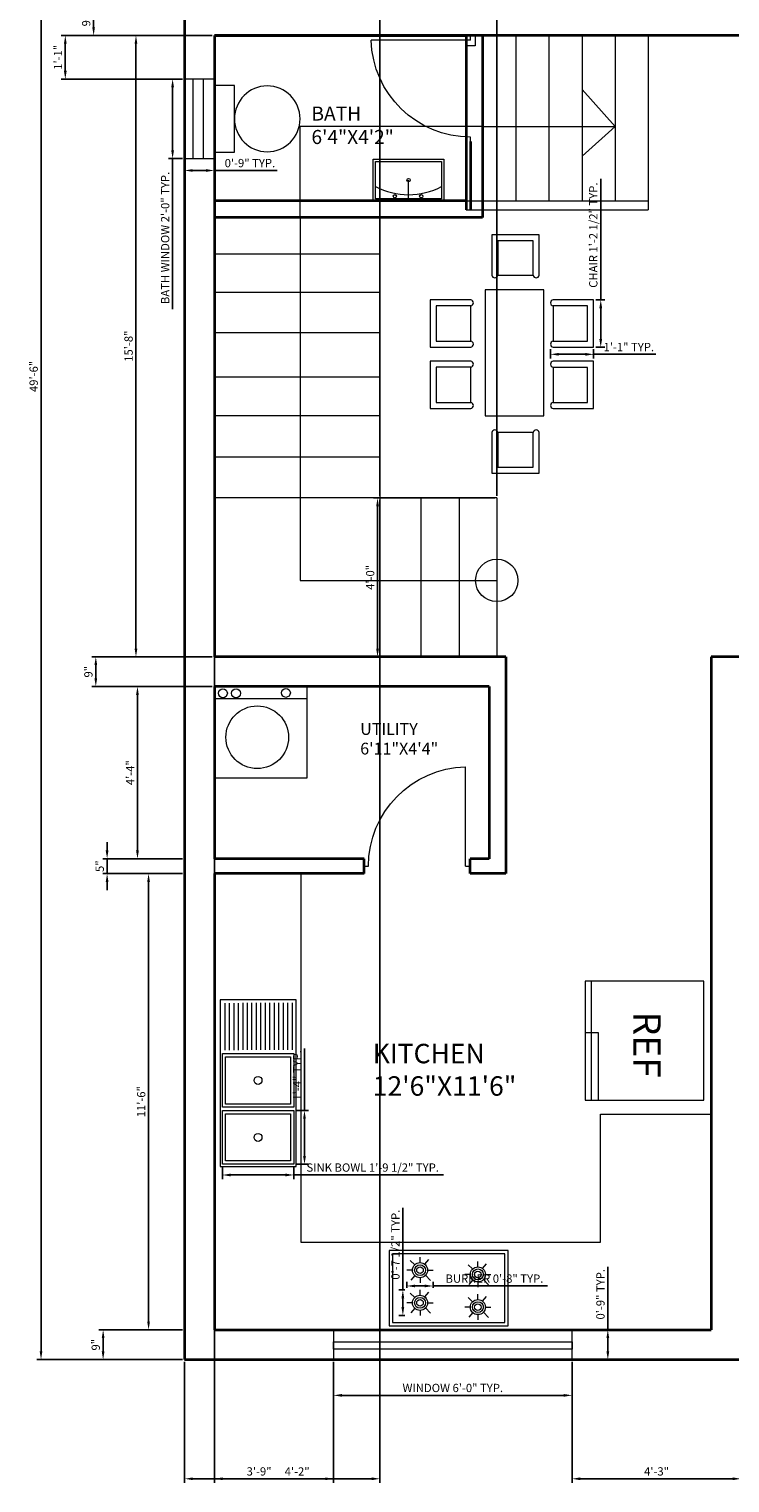
# Model space of a CAD drawing. Units: inches. Extents: x 808 to 1433, y 803 to 1556.
# Tile 1 of 4: x 808 to 1020, y 804 to 1243. Entities that reach past the tile are written whole.
import ezdxf

# ---------------------------------------------------------------- set-up
doc = ezdxf.new("R2010")
doc.units = ezdxf.units.IN
for name, color, linetype, lineweight in [('A-ANNO-DIMS', 7, 'Continuous', 13), ('A-AREA-IDEN', 7, 'Continuous', 18), ('A-FLOR-CASE', 7, 'Continuous', 18), ('A-FLOR-STRS', 7, 'Continuous', 18), ('A-WALL', 7, 'Continuous', 35)]:
    doc.layers.add(name, color=color, linetype=linetype, lineweight=lineweight)
for name, color, linetype, lineweight, true_color in [('A-ANNO-TEXT', 251, 'Continuous', 18, 0x636466), ('A-DOOR', 251, 'Continuous', 18, 0x636466), ('A-EQPM', 251, 'Continuous', 18, 0x636466), ('A-FIXT-PATT', 251, 'Continuous', 13, 0x636466), ('A-FLOR-FIXT', 251, 'Continuous', 18, 0x636466), ('A-FURN', 251, 'Continuous', 13, 0x636466), ('A-GLAZ', 251, 'Continuous', 18, 0x636466)]:
    doc.layers.add(name, color=color, linetype=linetype, lineweight=lineweight, true_color=true_color)
doc.styles.get("Standard").update_dxf_attribs({"font": 'arial.ttf'})
doc.dimstyles.new('ISO-25', dxfattribs={"dimtxt": 2.5, "dimasz": 2.5, "dimexe": 1.25, "dimexo": 0.625, "dimtad": 1, "dimdec": 0, "dimlunit": 3, "dimtxsty": 'Standard', "dimcen": 2.5, "dimadec": 0, "dimazin": 0, "dimtfac": 1, "dimtdec": 0, "dimtmove": 0, "dimatfit": 3, "dimfxl": 1, "dimarcsym": 0})

# ---------------------------------------------------------------- blocks, each defined once
blk = doc.blocks.new('*D12')
at = {"layer": 'A-ANNO-DIMS', "color": 0, "lineweight": -2, "transparency": 16777216}
for p, q in [((854.25, 1435.07), (810.3, 1435.07)), ((811.55, 1432.57), (811.55, 843.57)), ((854.25, 841.07), (810.3, 841.07))]:
    blk.add_line(p, q, dxfattribs=at)
at = {"layer": 'A-ANNO-DIMS', "color": 0, "transparency": 16777216}
for points in [[(811.14, 1432.57), (811.97, 1432.57), (811.55, 1435.07)], [(811.14, 843.57), (811.97, 843.57), (811.55, 841.07)]]:
    blk.add_solid(points, dxfattribs=at)
at = {"layer": 'Defpoints', "color": 0, "transparency": 16777216}
for p in [(854.88, 1435.07), (811.55, 841.07), (854.88, 841.07)]:
    blk.add_point(p, dxfattribs=at)
at = {"layer": 'A-ANNO-DIMS', "color": 0, "transparency": 16777216, "insert": (809.65, 1138.07), "char_height": 2.5, "attachment_point": 5, "rotation": 90}
blk.add_mtext('49\'-6"', dxfattribs=at)
blk = doc.blocks.new('*D15')
at = {"layer": 'A-ANNO-DIMS', "color": 0, "lineweight": -2, "transparency": 16777216}
for p, q in [((854.25, 1250.07), (826.18, 1250.07)), ((827.43, 1247.57), (827.43, 1243.57)), ((854.25, 1241.07), (826.18, 1241.07))]:
    blk.add_line(p, q, dxfattribs=at)
at = {"layer": 'A-ANNO-DIMS', "color": 0, "transparency": 16777216}
for points in [[(827.01, 1247.57), (827.84, 1247.57), (827.43, 1250.07)], [(827.01, 1243.57), (827.84, 1243.57), (827.43, 1241.07)]]:
    blk.add_solid(points, dxfattribs=at)
at = {"layer": 'Defpoints', "color": 0, "transparency": 16777216}
for p in [(854.88, 1250.07), (827.43, 1241.07), (854.88, 1241.07)]:
    blk.add_point(p, dxfattribs=at)
at = {"layer": 'A-ANNO-DIMS', "color": 0, "transparency": 16777216, "insert": (825.52, 1245.57), "char_height": 2.5, "attachment_point": 5, "rotation": 90}
blk.add_mtext('9"', dxfattribs=at)
blk = doc.blocks.new('*D16')
at = {"layer": 'A-ANNO-DIMS', "color": 0, "lineweight": -2, "transparency": 16777216}
for p, q in [((854.25, 1044.37), (839.42, 1044.37)), ((840.67, 1041.87), (840.67, 994.87)), ((854.25, 992.37), (839.42, 992.37))]:
    blk.add_line(p, q, dxfattribs=at)
at = {"layer": 'A-ANNO-DIMS', "color": 0, "transparency": 16777216}
for points in [[(840.25, 1041.87), (841.08, 1041.87), (840.67, 1044.37)], [(840.25, 994.87), (841.08, 994.87), (840.67, 992.37)]]:
    blk.add_solid(points, dxfattribs=at)
at = {"layer": 'Defpoints', "color": 0, "transparency": 16777216}
for p in [(854.88, 1044.37), (840.67, 992.37), (854.88, 992.37)]:
    blk.add_point(p, dxfattribs=at)
at = {"layer": 'A-ANNO-DIMS', "color": 0, "transparency": 16777216, "insert": (838.79, 1018.37), "char_height": 2.5, "attachment_point": 5, "rotation": 90}
blk.add_mtext('4\'-4"', dxfattribs=at)
blk = doc.blocks.new('*D17')
at = {"layer": 'A-ANNO-DIMS', "color": 0, "lineweight": -2, "transparency": 16777216}
for p, q in [((831.5, 994.87), (831.5, 997.37)), ((854.25, 992.37), (830.25, 992.37)), ((831.5, 992.37), (831.5, 987.87)), ((854.25, 987.87), (830.25, 987.87)), ((831.5, 985.37), (831.5, 982.87))]:
    blk.add_line(p, q, dxfattribs=at)
at = {"layer": 'A-ANNO-DIMS', "color": 0, "transparency": 16777216}
for points in [[(831.08, 994.87), (831.91, 994.87), (831.5, 992.37)], [(831.08, 985.37), (831.91, 985.37), (831.5, 987.87)]]:
    blk.add_solid(points, dxfattribs=at)
at = {"layer": 'Defpoints', "color": 0, "transparency": 16777216}
for p in [(854.88, 992.37), (831.5, 987.87), (854.88, 987.87)]:
    blk.add_point(p, dxfattribs=at)
at = {"layer": 'A-ANNO-DIMS', "color": 0, "transparency": 16777216, "insert": (829.6, 990.12), "char_height": 2.5, "attachment_point": 5, "rotation": 90}
blk.add_mtext('5"', dxfattribs=at)
blk = doc.blocks.new('*D18')
at = {"layer": 'A-ANNO-DIMS', "color": 0, "lineweight": -2, "transparency": 16777216}
for p, q in [((854.25, 987.87), (842.77, 987.87)), ((844.02, 985.37), (844.02, 852.57)), ((854.25, 850.07), (842.77, 850.07))]:
    blk.add_line(p, q, dxfattribs=at)
at = {"layer": 'A-ANNO-DIMS', "color": 0, "transparency": 16777216}
for points in [[(843.6, 985.37), (844.43, 985.37), (844.02, 987.87)], [(843.6, 852.57), (844.43, 852.57), (844.02, 850.07)]]:
    blk.add_solid(points, dxfattribs=at)
at = {"layer": 'Defpoints', "color": 0, "transparency": 16777216}
for p in [(854.88, 987.87), (844.02, 850.07), (854.88, 850.07)]:
    blk.add_point(p, dxfattribs=at)
at = {"layer": 'A-ANNO-DIMS', "color": 0, "transparency": 16777216, "insert": (842.12, 918.97), "char_height": 2.5, "attachment_point": 5, "rotation": 90}
blk.add_mtext('11\'-6"', dxfattribs=at)
blk = doc.blocks.new('*D19')
at = {"layer": 'A-ANNO-DIMS', "color": 0, "lineweight": -2, "transparency": 16777216}
for p, q in [((854.25, 850.07), (829.05, 850.07)), ((830.3, 847.57), (830.3, 843.57)), ((854.25, 841.07), (829.05, 841.07))]:
    blk.add_line(p, q, dxfattribs=at)
at = {"layer": 'A-ANNO-DIMS', "color": 0, "transparency": 16777216}
for points in [[(829.88, 847.57), (830.71, 847.57), (830.3, 850.07)], [(829.88, 843.57), (830.71, 843.57), (830.3, 841.07)]]:
    blk.add_solid(points, dxfattribs=at)
at = {"layer": 'Defpoints', "color": 0, "transparency": 16777216}
for p in [(854.88, 850.07), (830.3, 841.07), (854.88, 841.07)]:
    blk.add_point(p, dxfattribs=at)
at = {"layer": 'A-ANNO-DIMS', "color": 0, "transparency": 16777216, "insert": (828.39, 845.57), "char_height": 2.5, "attachment_point": 5, "rotation": 90}
blk.add_mtext('9"', dxfattribs=at)
blk = doc.blocks.new('*D27')
at = {"layer": 'A-ANNO-DIMS', "color": 0, "lineweight": -2, "transparency": 16777216}
for p, q in [((863.25, 1053.37), (826.84, 1053.37)), ((828.09, 1050.87), (828.09, 1046.87)), ((863.25, 1044.37), (826.84, 1044.37))]:
    blk.add_line(p, q, dxfattribs=at)
at = {"layer": 'A-ANNO-DIMS', "color": 0, "transparency": 16777216}
for points in [[(827.67, 1050.87), (828.5, 1050.87), (828.09, 1053.37)], [(827.67, 1046.87), (828.5, 1046.87), (828.09, 1044.37)]]:
    blk.add_solid(points, dxfattribs=at)
at = {"layer": 'Defpoints', "color": 0, "transparency": 16777216}
for p in [(863.88, 1053.37), (828.09, 1044.37), (863.88, 1044.37)]:
    blk.add_point(p, dxfattribs=at)
at = {"layer": 'A-ANNO-DIMS', "color": 0, "transparency": 16777216, "insert": (826.18, 1048.87), "char_height": 2.5, "attachment_point": 5, "rotation": 90}
blk.add_mtext('9"', dxfattribs=at)
blk = doc.blocks.new('*D28')
at = {"layer": 'A-ANNO-DIMS', "color": 0, "lineweight": -2, "transparency": 16777216}
for p, q in [((854.25, 1241.07), (838.97, 1241.07)), ((840.22, 1055.87), (840.22, 1238.57)), ((854.25, 1053.37), (838.97, 1053.37))]:
    blk.add_line(p, q, dxfattribs=at)
at = {"layer": 'A-ANNO-DIMS', "color": 0, "transparency": 16777216}
for points in [[(839.8, 1238.57), (840.63, 1238.57), (840.22, 1241.07)], [(839.8, 1055.87), (840.63, 1055.87), (840.22, 1053.37)]]:
    blk.add_solid(points, dxfattribs=at)
at = {"layer": 'Defpoints', "color": 0, "transparency": 16777216}
for p in [(840.22, 1241.07), (854.88, 1241.07), (854.88, 1053.37)]:
    blk.add_point(p, dxfattribs=at)
at = {"layer": 'A-ANNO-DIMS', "color": 0, "transparency": 16777216, "insert": (838.31, 1147.22), "char_height": 2.5, "attachment_point": 5, "rotation": 90}
blk.add_mtext('15\'-8"', dxfattribs=at)
blk = doc.blocks.new('WC')
blk.add_lwpolyline([(0, 19.84), (20.21, 19.84), (20.21, 25.9), (0, 25.9)], close=True)
for start, end in [(90, 270), (270, 90)]:
    blk.add_arc((10.11, 9.92), 9.92, start, end)
blk = doc.blocks.new('LAVATORY-COMPACT')
blk.add_line((10.66, 0.67), (10.66, 6.33))
for points in [[(21.33, 0), (0, 0), (0, 12.65), (21.33, 12.65)], [(20.66, 0.67), (0.67, 0.67), (0.67, 11.98), (20.66, 11.98)]]:
    blk.add_lwpolyline(points, close=True)
for centre in [(10.66, 6.33), (6.53, 1.45), (14.51, 1.45)]:
    blk.add_circle(centre, 0.492)
blk.add_arc((10.66, 23.6), 21.69, 242.5485, 297.4515)
blk = doc.blocks.new('COOKTOP-BURNER')
for p, q in [((2.4, 5.45), (1.03, 6.69)), ((3.99, 6.1), (3.99, 7.72)), ((5.4, 5.61), (6.63, 7.04)), ((1.71, 3.81), (0, 3.81)), ((2.42, 2.16), (1.25, 0.81)), ((3.99, 1.53), (3.99, 0)), ((5.67, 2.27), (7.14, 0.65)), ((6.27, 3.81), (7.92, 3.81))]:
    blk.add_line(p, q)
for radius in [2.28, 1.64, 0.989]:
    blk.add_circle((3.99, 3.81), radius)
blk = doc.blocks.new('WIN-72')
for points in [[(0, 0), (72, 0), (72, 9), (0, 9)], [(0, 5.39), (72, 5.39), (72, 3.12), (0, 3.12)]]:
    blk.add_lwpolyline(points, close=True)
blk = doc.blocks.new('WIN-24')
for p, q in [((0, 5.64), (24, 5.64)), ((0, 2.5), (24, 2.5))]:
    blk.add_line(p, q)
blk.add_lwpolyline([(0, 0), (24, 0), (24, 9), (0, 9)], close=True)
blk = doc.blocks.new('DOOR-32')
for p, q in [((1.38, 0), (1.38, 30)), ((1.38, 0), (0, 0)), ((32, 0), (30.69, 0))]:
    blk.add_line(p, q)
blk.add_arc((0.68, 0), 30.01, 0, 88.664)
blk = doc.blocks.new('CHAIR-DINING')
blk.add_lwpolyline([(0.77, 0), (13.02, 0), (13.02, 14.3), (0.77, 14.3)])
blk.add_lwpolyline([(0.77, 1.83), (11.19, 1.83), (11.19, 12.46), (0.77, 12.46)], close=True)
for centre in [(0.93, 13.38), (0.93, 0.92)]:
    blk.add_arc(centre, 0.932, 100.176, 259.824)
blk = doc.blocks.new('SINK-BOWL')
for points in [[(21.57, 0), (0, 0), (0, 16.24), (21.57, 16.24)], [(20.57, 1), (1, 1), (1, 15.24), (20.57, 15.24)]]:
    blk.add_lwpolyline(points, close=True)
blk.add_circle((10.78, 8.12), 1.19)
blk = doc.blocks.new('*D41')
at = {"layer": 'A-ANNO-DIMS', "color": 0, "lineweight": -2, "transparency": 16777216}
for p, q in [((899.87, 840.44), (899.87, 829.02)), ((971.87, 840.44), (971.87, 829.02)), ((902.37, 830.27), (969.37, 830.27))]:
    blk.add_line(p, q, dxfattribs=at)
at = {"layer": 'A-ANNO-DIMS', "color": 0, "transparency": 16777216}
for points in [[(902.37, 830.68), (902.37, 829.85), (899.87, 830.27)], [(969.37, 830.68), (969.37, 829.85), (971.87, 830.27)]]:
    blk.add_solid(points, dxfattribs=at)
at = {"layer": 'Defpoints', "color": 0, "transparency": 16777216}
for p in [(899.87, 841.07), (971.87, 841.07), (971.87, 830.27)]:
    blk.add_point(p, dxfattribs=at)
at = {"layer": 'A-ANNO-DIMS', "color": 0, "transparency": 16777216, "insert": (935.87, 832.18), "char_height": 2.5, "attachment_point": 5}
blk.add_mtext('WINDOW 6\'-0" TYP.', dxfattribs=at)
blk = doc.blocks.new('*D42')
at = {"layer": 'A-ANNO-DIMS', "color": 0, "lineweight": -2, "transparency": 16777216}
for p, q in [((982.67, 850.07), (982.67, 869.05)), ((972.5, 850.07), (983.92, 850.07)), ((982.67, 843.57), (982.67, 847.57)), ((972.5, 841.07), (983.92, 841.07))]:
    blk.add_line(p, q, dxfattribs=at)
at = {"layer": 'A-ANNO-DIMS', "color": 0, "transparency": 16777216}
for points in [[(982.25, 847.57), (983.09, 847.57), (982.67, 850.07)], [(982.25, 843.57), (983.09, 843.57), (982.67, 841.07)]]:
    blk.add_solid(points, dxfattribs=at)
at = {"layer": 'Defpoints', "color": 0, "transparency": 16777216}
for p in [(971.87, 850.07), (982.67, 850.07), (971.87, 841.07)]:
    blk.add_point(p, dxfattribs=at)
at = {"layer": 'A-ANNO-DIMS', "color": 0, "transparency": 16777216, "insert": (980.77, 860.81), "char_height": 2.5, "attachment_point": 5, "rotation": 90}
blk.add_mtext('0\'-9" TYP.', dxfattribs=at)
blk = doc.blocks.new('*D43')
at = {"layer": 'A-ANNO-DIMS', "color": 0, "lineweight": -2, "transparency": 16777216}
for p, q in [((854.25, 1227.89), (850.03, 1227.89)), ((851.28, 1225.39), (851.28, 1206.39)), ((854.25, 1203.89), (850.03, 1203.89)), ((851.28, 1203.89), (851.28, 1158.43))]:
    blk.add_line(p, q, dxfattribs=at)
at = {"layer": 'A-ANNO-DIMS', "color": 0, "transparency": 16777216}
for points in [[(850.86, 1225.39), (851.7, 1225.39), (851.28, 1227.89)], [(850.86, 1206.39), (851.7, 1206.39), (851.28, 1203.89)]]:
    blk.add_solid(points, dxfattribs=at)
at = {"layer": 'Defpoints', "color": 0, "transparency": 16777216}
for p in [(854.88, 1227.89), (851.28, 1203.89), (854.88, 1203.89)]:
    blk.add_point(p, dxfattribs=at)
at = {"layer": 'A-ANNO-DIMS', "color": 0, "transparency": 16777216, "insert": (849.36, 1179.91), "char_height": 2.5, "attachment_point": 5, "rotation": 90}
blk.add_mtext('BATH WINDOW 2\'-0" TYP.', dxfattribs=at)
blk = doc.blocks.new('*D44')
at = {"layer": 'A-ANNO-DIMS', "color": 0, "lineweight": -2, "transparency": 16777216}
for p, q in [((854.88, 1203.26), (854.88, 1199.04)), ((857.38, 1200.29), (861.38, 1200.29)), ((863.88, 1203.26), (863.88, 1199.04)), ((863.88, 1200.29), (882.87, 1200.29))]:
    blk.add_line(p, q, dxfattribs=at)
at = {"layer": 'A-ANNO-DIMS', "color": 0, "transparency": 16777216}
for points in [[(857.38, 1200.7), (857.38, 1199.87), (854.88, 1200.29)], [(861.38, 1200.7), (861.38, 1199.87), (863.88, 1200.29)]]:
    blk.add_solid(points, dxfattribs=at)
at = {"layer": 'Defpoints', "color": 0, "transparency": 16777216}
for p in [(854.88, 1203.89), (863.88, 1203.89), (863.88, 1200.29)]:
    blk.add_point(p, dxfattribs=at)
at = {"layer": 'A-ANNO-DIMS', "color": 0, "transparency": 16777216, "insert": (874.62, 1202.19), "char_height": 2.5, "attachment_point": 5}
blk.add_mtext('0\'-9" TYP.', dxfattribs=at)
blk = doc.blocks.new('*D59')
at = {"layer": 'A-ANNO-DIMS', "color": 0, "lineweight": -2, "transparency": 16777216}
for p, q in [((980.53, 1161.19), (980.53, 1197.81)), ((979.01, 1161.19), (981.78, 1161.19)), ((980.53, 1149.4), (980.53, 1158.69)), ((979.01, 1146.9), (981.78, 1146.9))]:
    blk.add_line(p, q, dxfattribs=at)
at = {"layer": 'A-ANNO-DIMS', "color": 0, "transparency": 16777216}
for points in [[(980.11, 1158.69), (980.95, 1158.69), (980.53, 1161.19)], [(980.11, 1149.4), (980.95, 1149.4), (980.53, 1146.9)]]:
    blk.add_solid(points, dxfattribs=at)
at = {"layer": 'Defpoints', "color": 0, "transparency": 16777216}
for p in [(978.39, 1161.19), (980.53, 1161.19), (978.39, 1146.9)]:
    blk.add_point(p, dxfattribs=at)
at = {"layer": 'A-ANNO-DIMS', "color": 0, "transparency": 16777216, "insert": (978.61, 1180.75), "char_height": 2.5, "attachment_point": 5, "rotation": 90}
blk.add_mtext('CHAIR 1\'-2 1/2" TYP.', dxfattribs=at)
blk = doc.blocks.new('*D60')
at = {"layer": 'A-ANNO-DIMS', "color": 0, "lineweight": -2, "transparency": 16777216}
for p, q in [((965.37, 1146.27), (965.37, 1143.5)), ((967.87, 1144.75), (975.89, 1144.75)), ((978.39, 1146.27), (978.39, 1143.5)), ((978.39, 1144.75), (997.14, 1144.75))]:
    blk.add_line(p, q, dxfattribs=at)
at = {"layer": 'A-ANNO-DIMS', "color": 0, "transparency": 16777216}
for points in [[(967.87, 1145.17), (967.87, 1144.33), (965.37, 1144.75)], [(975.89, 1145.17), (975.89, 1144.33), (978.39, 1144.75)]]:
    blk.add_solid(points, dxfattribs=at)
at = {"layer": 'Defpoints', "color": 0, "transparency": 16777216}
for p in [(965.37, 1146.9), (978.39, 1146.9), (978.39, 1144.75)]:
    blk.add_point(p, dxfattribs=at)
at = {"layer": 'A-ANNO-DIMS', "color": 0, "transparency": 16777216, "insert": (989.01, 1146.63), "char_height": 2.5, "attachment_point": 5}
blk.add_mtext('1\'-1" TYP.', dxfattribs=at)
blk = doc.blocks.new('*D61')
at = {"layer": 'A-ANNO-DIMS', "color": 0, "lineweight": -2, "transparency": 16777216}
for p, q in [((866.29, 899.45), (866.29, 895.59)), ((868.79, 896.84), (885.35, 896.84)), ((887.85, 899.45), (887.85, 895.59)), ((887.85, 896.84), (933.03, 896.84))]:
    blk.add_line(p, q, dxfattribs=at)
at = {"layer": 'A-ANNO-DIMS', "color": 0, "transparency": 16777216}
for points in [[(868.79, 897.26), (868.79, 896.42), (866.29, 896.84)], [(885.35, 897.26), (885.35, 896.42), (887.85, 896.84)]]:
    blk.add_solid(points, dxfattribs=at)
at = {"layer": 'Defpoints', "color": 0, "transparency": 16777216}
for p in [(866.29, 900.07), (887.85, 900.07), (887.85, 896.84)]:
    blk.add_point(p, dxfattribs=at)
at = {"layer": 'A-ANNO-DIMS', "color": 0, "transparency": 16777216, "insert": (911.69, 898.76), "char_height": 2.5, "attachment_point": 5}
blk.add_mtext('SINK BOWL 1\'-9 1/2" TYP.', dxfattribs=at)
blk = doc.blocks.new('*D62')
at = {"layer": 'A-ANNO-DIMS', "color": 0, "lineweight": -2, "transparency": 16777216}
for p, q in [((891.09, 916.31), (891.09, 935.07)), ((888.48, 916.31), (892.34, 916.31)), ((891.09, 902.57), (891.09, 913.81)), ((888.48, 900.07), (892.34, 900.07))]:
    blk.add_line(p, q, dxfattribs=at)
at = {"layer": 'A-ANNO-DIMS', "color": 0, "transparency": 16777216}
for points in [[(890.67, 913.81), (891.51, 913.81), (891.09, 916.31)], [(890.67, 902.57), (891.51, 902.57), (891.09, 900.07)]]:
    blk.add_solid(points, dxfattribs=at)
at = {"layer": 'Defpoints', "color": 0, "transparency": 16777216}
for p in [(887.85, 916.31), (891.09, 916.31), (887.85, 900.07)]:
    blk.add_point(p, dxfattribs=at)
at = {"layer": 'A-ANNO-DIMS', "color": 0, "transparency": 16777216, "insert": (889.21, 926.94), "char_height": 2.5, "attachment_point": 5, "rotation": 90}
blk.add_mtext('1\'-4" TYP.', dxfattribs=at)
blk = doc.blocks.new('*D63')
at = {"layer": 'A-ANNO-DIMS', "color": 0, "lineweight": -2, "transparency": 16777216}
for p, q in [((921.98, 862.75), (921.98, 864.56)), ((924.48, 863.31), (927.4, 863.31)), ((929.9, 862.75), (929.9, 864.56)), ((929.9, 863.31), (964.49, 863.31))]:
    blk.add_line(p, q, dxfattribs=at)
at = {"layer": 'A-ANNO-DIMS', "color": 0, "transparency": 16777216}
for points in [[(924.48, 863.73), (924.48, 862.9), (921.98, 863.31)], [(927.4, 863.73), (927.4, 862.9), (929.9, 863.31)]]:
    blk.add_solid(points, dxfattribs=at)
at = {"layer": 'Defpoints', "color": 0, "transparency": 16777216}
for p in [(921.98, 862.12), (929.9, 863.31), (929.9, 862.12)]:
    blk.add_point(p, dxfattribs=at)
at = {"layer": 'A-ANNO-DIMS', "color": 0, "transparency": 16777216, "insert": (948.44, 865.21), "char_height": 2.5, "attachment_point": 5}
blk.add_mtext('BURNER 0\'-8" TYP.', dxfattribs=at)
blk = doc.blocks.new('*D64')
at = {"layer": 'A-ANNO-DIMS', "color": 0, "lineweight": -2, "transparency": 16777216}
for p, q in [((920.79, 862.12), (920.79, 886.94)), ((921.35, 862.12), (919.54, 862.12)), ((920.79, 856.91), (920.79, 859.62)), ((921.35, 854.41), (919.54, 854.41))]:
    blk.add_line(p, q, dxfattribs=at)
at = {"layer": 'A-ANNO-DIMS', "color": 0, "transparency": 16777216}
for points in [[(920.37, 859.62), (921.2, 859.62), (920.79, 862.12)], [(920.37, 856.91), (921.2, 856.91), (920.79, 854.41)]]:
    blk.add_solid(points, dxfattribs=at)
at = {"layer": 'Defpoints', "color": 0, "transparency": 16777216}
for p in [(920.79, 862.12), (921.98, 862.12), (921.98, 854.41)]:
    blk.add_point(p, dxfattribs=at)
at = {"layer": 'A-ANNO-DIMS', "color": 0, "transparency": 16777216, "insert": (918.87, 875.78), "char_height": 2.5, "attachment_point": 5, "rotation": 90}
blk.add_mtext('0\'-7 1/2" TYP.', dxfattribs=at)
blk = doc.blocks.new('*D65')
at = {"layer": 'A-ANNO-DIMS', "color": 0, "lineweight": -2, "transparency": 16777216}
for p, q in [((854.88, 840.44), (854.88, 803.82)), ((899.87, 840.44), (899.87, 803.82)), ((857.38, 805.07), (897.37, 805.07))]:
    blk.add_line(p, q, dxfattribs=at)
at = {"layer": 'A-ANNO-DIMS', "color": 0, "transparency": 16777216}
for points in [[(857.38, 805.48), (857.38, 804.65), (854.88, 805.07)], [(897.37, 805.48), (897.37, 804.65), (899.87, 805.07)]]:
    blk.add_solid(points, dxfattribs=at)
at = {"layer": 'Defpoints', "color": 0, "transparency": 16777216}
for p in [(854.88, 841.07), (899.87, 841.07), (899.87, 805.07)]:
    blk.add_point(p, dxfattribs=at)
at = {"layer": 'A-ANNO-DIMS', "color": 0, "transparency": 16777216, "insert": (877.38, 806.97), "char_height": 2.5, "attachment_point": 5}
blk.add_mtext('3\'-9"', dxfattribs=at)
blk = doc.blocks.new('*D66')
at = {"layer": 'A-ANNO-DIMS', "color": 0, "lineweight": -2, "transparency": 16777216}
for p, q in [((1022.88, 849.44), (1022.88, 803.82)), ((971.87, 840.44), (971.87, 803.82)), ((974.37, 805.07), (1020.38, 805.07))]:
    blk.add_line(p, q, dxfattribs=at)
at = {"layer": 'A-ANNO-DIMS', "color": 0, "transparency": 16777216}
for points in [[(974.37, 805.48), (974.37, 804.65), (971.87, 805.07)], [(1020.38, 805.48), (1020.38, 804.65), (1022.88, 805.07)]]:
    blk.add_solid(points, dxfattribs=at)
at = {"layer": 'Defpoints', "color": 0, "transparency": 16777216}
for p in [(1022.88, 850.07), (971.87, 841.07), (1022.88, 805.07)]:
    blk.add_point(p, dxfattribs=at)
at = {"layer": 'A-ANNO-DIMS', "color": 0, "transparency": 16777216, "insert": (997.38, 806.97), "char_height": 2.5, "attachment_point": 5}
blk.add_mtext('4\'-3"', dxfattribs=at)
blk = doc.blocks.new('*D75')
at = {"layer": 'A-ANNO-DIMS', "color": 0, "lineweight": -2, "transparency": 16777216}
for p, q in [((863.25, 1241.07), (817.63, 1241.07)), ((818.88, 1238.57), (818.88, 1230.39)), ((854.25, 1227.89), (817.63, 1227.89))]:
    blk.add_line(p, q, dxfattribs=at)
at = {"layer": 'A-ANNO-DIMS', "color": 0, "transparency": 16777216}
for points in [[(818.46, 1238.57), (819.3, 1238.57), (818.88, 1241.07)], [(818.46, 1230.39), (819.3, 1230.39), (818.88, 1227.89)]]:
    blk.add_solid(points, dxfattribs=at)
at = {"layer": 'Defpoints', "color": 0, "transparency": 16777216}
for p in [(863.88, 1241.07), (818.88, 1227.89), (854.88, 1227.89)]:
    blk.add_point(p, dxfattribs=at)
at = {"layer": 'A-ANNO-DIMS', "color": 0, "transparency": 16777216, "insert": (817, 1234.48), "char_height": 2.5, "attachment_point": 5, "rotation": 90}
blk.add_mtext('1\'-1"', dxfattribs=at)
blk = doc.blocks.new('*D76')
at = {"layer": 'A-ANNO-DIMS', "color": 0, "lineweight": -2, "transparency": 16777216}
for p, q in [((863.88, 1100.75), (863.88, 803.82)), ((913.88, 1100.75), (913.88, 803.82)), ((866.38, 805.07), (911.38, 805.07))]:
    blk.add_line(p, q, dxfattribs=at)
at = {"layer": 'A-ANNO-DIMS', "color": 0, "transparency": 16777216}
for points in [[(866.38, 805.48), (866.38, 804.65), (863.88, 805.07)], [(911.38, 805.48), (911.38, 804.65), (913.88, 805.07)]]:
    blk.add_solid(points, dxfattribs=at)
at = {"layer": 'Defpoints', "color": 0, "transparency": 16777216}
for p in [(863.88, 1101.37), (913.88, 1101.37), (913.88, 805.07)]:
    blk.add_point(p, dxfattribs=at)
at = {"layer": 'A-ANNO-DIMS', "color": 0, "transparency": 16777216, "insert": (888.88, 806.95), "char_height": 2.5, "attachment_point": 5}
blk.add_mtext('4\'-2"', dxfattribs=at)
blk = doc.blocks.new('*D77')
at = {"layer": 'A-ANNO-DIMS', "color": 0, "lineweight": -2, "transparency": 16777216}
for p, q in [((948.53, 1101.37), (911.9, 1101.37)), ((913.15, 1055.87), (913.15, 1098.87)), ((948.53, 1053.37), (911.9, 1053.37))]:
    blk.add_line(p, q, dxfattribs=at)
at = {"layer": 'A-ANNO-DIMS', "color": 0, "transparency": 16777216}
for points in [[(912.73, 1098.87), (913.57, 1098.87), (913.15, 1101.37)], [(912.73, 1055.87), (913.57, 1055.87), (913.15, 1053.37)]]:
    blk.add_solid(points, dxfattribs=at)
at = {"layer": 'Defpoints', "color": 0, "transparency": 16777216}
for p in [(913.15, 1101.37), (949.15, 1101.37), (949.15, 1053.37)]:
    blk.add_point(p, dxfattribs=at)
at = {"layer": 'A-ANNO-DIMS', "color": 0, "transparency": 16777216, "insert": (911.25, 1077.37), "char_height": 2.5, "attachment_point": 5, "rotation": 90}
blk.add_mtext('4\'-0"', dxfattribs=at)
blk = doc.blocks.new('*D78')
at = {"layer": 'A-ANNO-DIMS', "color": 0, "lineweight": -2, "transparency": 16777216}
for p, q in [((913.88, 1102), (913.88, 1472.32)), ((949.15, 1102), (949.15, 1472.32)), ((916.38, 1471.07), (946.65, 1471.07))]:
    blk.add_line(p, q, dxfattribs=at)
at = {"layer": 'A-ANNO-DIMS', "color": 0, "transparency": 16777216}
for points in [[(916.38, 1471.48), (916.38, 1470.65), (913.88, 1471.07)], [(946.65, 1471.48), (946.65, 1470.65), (949.15, 1471.07)]]:
    blk.add_solid(points, dxfattribs=at)
at = {"layer": 'Defpoints', "color": 0, "transparency": 16777216}
for p in [(949.15, 1471.07), (913.88, 1101.37), (949.15, 1101.37)]:
    blk.add_point(p, dxfattribs=at)
at = {"layer": 'A-ANNO-DIMS', "color": 0, "transparency": 16777216, "insert": (931.51, 1472.98), "char_height": 2.5, "attachment_point": 5}
blk.add_mtext('2\'-11 1/2"', dxfattribs=at)

msp = doc.modelspace()

# ---------------------------------------------------------------- hatches: boundary and pattern name
at = {"layer": 'A-FIXT-PATT'}
h = msp.add_hatch(dxfattribs=at)
h.set_pattern_fill('ANSI31', color=256, scale=0.426729, angle=45, style=0)
h.paths.add_polyline_path([(866.42, 934.55), (871.91, 934.55), (871.91, 934.66), (887.92, 934.66), (887.92, 948.86), (871.91, 948.86), (871.91, 948.76), (866.42, 948.76)])

# ---------------------------------------------------------------- linework, layer by layer
at = {"layer": 'A-DOOR'}
msp.add_lwpolyline([(939.88, 1241.07), (942.62, 1241.07), (942.62, 1237.91), (939.88, 1237.91)], close=True, dxfattribs=at)
at = {"layer": 'A-EQPM'}
for p, q in [((863.88, 1040.78), (891.83, 1040.78)), ((977.76, 919.4), (977.76, 955.4)), ((952.61, 874.07), (916.62, 874.07)), ((916.62, 874.07), (916.62, 851.24)), ((952.61, 851.24), (952.61, 874.07)), ((951.61, 873.07), (917.62, 873.07)), ((917.62, 873.07), (917.62, 852.24)), ((951.61, 852.24), (951.61, 873.07)), ((917.62, 852.24), (951.61, 852.24)), ((916.62, 851.24), (952.61, 851.24))]:
    msp.add_line(p, q, dxfattribs=at)
for points in [[(863.88, 1044.37), (891.83, 1044.37), (891.83, 1016.75), (863.88, 1016.75)], [(975.85, 919.4), (1011.67, 919.4), (1011.67, 955.4), (975.85, 955.4)], [(975.85, 919.4), (979.85, 919.4), (979.85, 939.76), (975.85, 939.76)]]:
    msp.add_lwpolyline(points, close=True, dxfattribs=at)
for centre, radius in [((866.45, 1042.37), 1.35), ((870.42, 1042.35), 1.35), ((885.47, 1042.48), 1.35), ((876.83, 1029.08), 9.46)]:
    msp.add_circle(centre, radius, dxfattribs=at)
at = {"layer": 'A-FLOR-CASE'}
for p, q in [((889.94, 987.87), (889.94, 876.52)), ((980.47, 876.52), (980.47, 915.21)), ((980.47, 915.21), (1013.88, 915.21)), ((889.94, 876.52), (980.47, 876.52))]:
    msp.add_line(p, q, dxfattribs=at)
at = {"layer": 'A-FLOR-FIXT'}
for p, q in [((888.6, 949.77), (865.6, 949.77)), ((865.6, 949.77), (865.6, 899.39)), ((888.6, 899.39), (888.6, 949.77)), ((865.6, 899.39), (888.6, 899.39))]:
    msp.add_line(p, q, dxfattribs=at)
at = {"layer": 'A-FLOR-STRS'}
for p, q in [((944.88, 1241.07), (944.88, 1191.07)), ((954.88, 1241.07), (954.88, 1191.07)), ((964.88, 1241.07), (964.88, 1191.07)), ((974.88, 1241.07), (974.88, 1191.07)), ((984.88, 1241.07), (984.88, 1191.07)), ((994.88, 1241.07), (994.88, 1188.43)), ((984.88, 1213.57), (974.88, 1224.76)), ((889.83, 1186.07), (889.83, 1213.57)), ((944.88, 1213.57), (889.83, 1213.57)), ((944.88, 1213.57), (984.88, 1213.57)), ((984.88, 1213.57), (974.88, 1204.63)), ((939.88, 1191.07), (994.88, 1191.07)), ((889.83, 1186.07), (889.83, 1076.45)), ((913.88, 1186.07), (913.88, 1101.37)), ((939.88, 1188.43), (994.88, 1188.43)), ((863.88, 1175.09), (913.88, 1175.09)), ((863.88, 1163.56), (913.88, 1163.56)), ((863.88, 1151.34), (913.88, 1151.34)), ((863.88, 1137.98), (913.88, 1137.98)), ((863.88, 1126.25), (913.88, 1126.25)), ((863.88, 1113.83), (913.88, 1113.83)), ((949.15, 1101.37), (863.88, 1101.37)), ((913.88, 1101.37), (913.88, 1053.37)), ((926.22, 1101.37), (926.22, 1053.37)), ((937.77, 1101.37), (937.77, 1053.37)), ((949.15, 1101.37), (949.15, 1053.37)), ((889.83, 1076.45), (949.15, 1076.45))]:
    msp.add_line(p, q, dxfattribs=at)
msp.add_circle((949.15, 1076.45), 6.4, dxfattribs=at)
at = {"layer": 'A-FURN'}
msp.add_lwpolyline([(945.59, 1126.12), (963.35, 1126.12), (963.35, 1164.24), (945.59, 1164.24)], close=True, dxfattribs=at)
at = {"layer": 'A-WALL'}
for p, q in [((854.88, 1435.07), (854.88, 841.07)), ((863.88, 1241.07), (863.88, 1053.37)), ((863.88, 1241.07), (939.88, 1241.07)), ((1023.88, 1241.07), (863.88, 1241.07)), ((939.88, 1241.07), (939.88, 1188.43)), ((944.88, 1241.07), (944.88, 1186.07)), ((941.25, 1209.07), (941.25, 1188.43)), ((939.88, 1191.07), (863.88, 1191.07)), ((944.88, 1186.07), (863.88, 1186.07)), ((951.88, 1053.37), (863.88, 1053.37)), ((951.88, 1053.37), (951.88, 987.87)), ((1013.88, 1053.37), (1013.88, 850.07)), ((1022.88, 1053.37), (1013.88, 1053.37)), ((863.88, 1044.37), (863.88, 992.37)), ((946.88, 1044.37), (863.88, 1044.37)), ((946.88, 1044.37), (946.88, 992.37)), ((909.07, 992.37), (863.88, 992.37)), ((909.07, 987.87), (909.07, 992.37)), ((946.88, 992.37), (941.07, 992.37)), ((941.07, 987.87), (941.07, 992.37)), ((863.88, 987.87), (863.88, 850.07)), ((909.07, 987.87), (863.88, 987.87)), ((951.88, 987.87), (941.07, 987.87)), ((863.88, 850.07), (1013.88, 850.07)), ((854.88, 841.07), (1380.88, 841.07))]:
    msp.add_line(p, q, dxfattribs=at)

# ---------------------------------------------------------------- block references
at = {"layer": 'A-DOOR', "extrusion": (0, 0, -1), "zscale": -1, "rotation": 269.9999999999882}
msp.add_blockref('DOOR-32', (-941.25, 1241.07), dxfattribs=at)
at = {"layer": 'A-DOOR', "extrusion": (0, 0, -1), "zscale": -1}
msp.add_blockref('DOOR-32', (-941.07, 990.12), dxfattribs=at)
at = {"layer": 'A-EQPM'}
for p in [(921.98, 864.27), (939.46, 862.99), (921.98, 854.41), (939.46, 853.12)]:
    msp.add_blockref('COOKTOP-BURNER', p, dxfattribs=at)
at = {"layer": 'A-FLOR-FIXT', "rotation": 90.0000000000017}
msp.add_blockref('WC', (889.78, 1205.78), dxfattribs=at)
at = {"layer": 'A-FLOR-FIXT'}
for name, p in [('LAVATORY-COMPACT', (911.84, 1191.07)), ('SINK-BOWL', (866.29, 917.28)), ('SINK-BOWL', (866.29, 900.07))]:
    msp.add_blockref(name, p, dxfattribs=at)
at = {"layer": 'A-FURN'}
for p, rotation in [((961.93, 1167.86), 90.0000000000036), ((942.07, 1161.23), 180), ((942.07, 1142.69), 180), ((947.63, 1121.9), 270.0000000000008)]:
    msp.add_blockref('CHAIR-DINING', p, dxfattribs=dict(at, rotation=rotation))
for p in [(965.37, 1146.89), (965.37, 1128.36)]:
    msp.add_blockref('CHAIR-DINING', p, dxfattribs=at)
at = {"layer": 'A-GLAZ', "rotation": 270.0000000000003}
msp.add_blockref('WIN-24', (854.88, 1227.89), dxfattribs=at)
at = {"layer": 'A-GLAZ'}
msp.add_blockref('WIN-72', (899.87, 841.07), dxfattribs=at)

# ---------------------------------------------------------------- texts
at = {"layer": 'A-ANNO-TEXT', "insert": (998.64, 946.2), "char_height": 8.255, "attachment_point": 1, "rotation": 270}
msp.add_mtext_dynamic_manual_height_columns('REF', width=135.578, gutter_width=41.27, heights=[0], dxfattribs=at)
at = {"layer": 'A-AREA-IDEN', "attachment_point": 1}
for s, width, gutter_width, insert, char_height in [('BATH\\P6\'4"X4\'2"', 49.0046, 21.22, (893.19, 1219.6), 4.243), ('UTILITY\\P6\'11"X4\'4"', 37.4104, 17.79, (907.91, 1033.35), 3.559), ('KITCHEN\\P12\'6"X11\'6"', 117.6336, 29.39, (911.69, 936.46), 5.8788)]:
    msp.add_mtext_dynamic_manual_height_columns(s, width=width, gutter_width=gutter_width, heights=[0], dxfattribs=dict(at, insert=insert, char_height=char_height))

# ---------------------------------------------------------------- dimensions: what is measured, and where the dimension line sits
at = {"layer": 'A-ANNO-DIMS'}
for base, p1, p2, picture, middle in [((949.15, 1471.07), (913.88, 1101.37), (949.15, 1101.37), '*D78', (931.51, 1472.98)), ((913.88, 805.07), (863.88, 1101.37), (913.88, 1101.37), '*D76', (888.88, 806.95)), ((1022.88, 805.07), (971.87, 841.07), (1022.88, 850.07), '*D66', (997.38, 806.97)), ((899.87, 805.07), (854.88, 841.07), (899.87, 841.07), '*D65', (877.38, 806.97))]:
    dim = msp.add_linear_dim(base=base, p1=p1, p2=p2, dimstyle='ISO-25', override={"dimdec": 1, "dimlfac": 1, "dimrnd": 0, "dimzin": 1, "dimdsep": 46, "dimlunit": 4, "dimfrac": 2}, dxfattribs=at)
    dim.commit()
    dim.dimension.update_dxf_attribs({"geometry": picture, "text_midpoint": middle})
for base, p1, p2, override, picture, middle in [((811.55, 841.07), (854.88, 1435.07), (854.88, 841.07), {"dimclrd": 0, "dimclre": 0, "dimclrt": 0}, '*D12', (809.65, 1138.07)), ((827.43, 1241.07), (854.88, 1250.07), (854.88, 1241.07), {"dimclrd": 0, "dimclre": 0, "dimclrt": 0}, '*D15', (825.52, 1245.57)), ((818.88, 1227.89), (863.88, 1241.07), (854.88, 1227.89), {"dimdec": 1, "dimlfac": 1, "dimrnd": 0, "dimzin": 1, "dimdsep": 46, "dimlunit": 4, "dimfrac": 2}, '*D75', (817, 1234.48)), ((840.22, 1241.07), (854.88, 1053.37), (854.88, 1241.07), {"dimclrd": 0, "dimclre": 0, "dimclrt": 0}, '*D28', (838.31, 1147.22)), ((913.15, 1101.37), (949.15, 1053.37), (949.15, 1101.37), {"dimdec": 1, "dimlfac": 1, "dimrnd": 0, "dimzin": 1, "dimdsep": 46, "dimlunit": 4, "dimfrac": 2}, '*D77', (911.25, 1077.37)), ((828.09, 1044.37), (863.88, 1053.37), (863.88, 1044.37), {"dimclrd": 0, "dimclre": 0, "dimclrt": 0}, '*D27', (826.18, 1048.87)), ((840.67, 992.37), (854.88, 1044.37), (854.88, 992.37), {"dimclrd": 0, "dimclre": 0, "dimclrt": 0}, '*D16', (838.79, 1018.37)), ((831.49731928, 987.87144282), (854.87953788, 992.37144282), (854.87953788, 987.87144282), {"dimclrd": 0, "dimclre": 0, "dimclrt": 0}, '*D17', (829.60100277, 990.12144282)), ((844.02, 850.07), (854.88, 987.87), (854.88, 850.07), {"dimclrd": 0, "dimclre": 0, "dimclrt": 0}, '*D18', (842.12, 918.97)), ((830.3, 841.07), (854.88, 850.07), (854.88, 841.07), {"dimclrd": 0, "dimclre": 0, "dimclrt": 0}, '*D19', (828.39, 845.57))]:
    dim = msp.add_linear_dim(base=base, p1=p1, p2=p2, angle=90, dimstyle='ISO-25', override=override, dxfattribs=at)
    dim.commit()
    dim.dimension.update_dxf_attribs({"geometry": picture, "text_midpoint": middle})
for base, p1, p2, angle, text, picture, middle in [((851.28, 1203.89), (854.88, 1227.89), (854.88, 1203.89), 270, 'BATH WINDOW <> TYP.', '*D43', (849.36, 1179.91)), ((980.53, 1161.19), (978.39, 1146.9), (978.39, 1161.19), 90, 'CHAIR <> TYP.', '*D59', (978.61, 1180.75)), ((891.09, 916.31), (887.85, 900.07), (887.85, 916.31), 90, '<> TYP.', '*D62', (889.21, 926.94)), ((920.79, 862.12), (921.98, 854.41), (921.98, 862.12), 90, '<> TYP.', '*D64', (918.87, 875.78)), ((982.67, 850.07), (971.87, 841.07), (971.87, 850.07), 90, '<> TYP.', '*D42', (980.77, 860.81))]:
    dim = msp.add_linear_dim(base=base, p1=p1, p2=p2, angle=angle, text=text, dimstyle='ISO-25', override={"dimdec": 1, "dimlfac": 1, "dimrnd": 0, "dimzin": 1, "dimdsep": 46, "dimlunit": 4, "dimfrac": 2}, dxfattribs=at)
    dim.commit()
    dim.dimension.update_dxf_attribs({"geometry": picture, "text_midpoint": middle})
for base, p1, p2, text, picture, middle in [((863.88, 1200.29), (854.88, 1203.89), (863.88, 1203.89), '<> TYP.', '*D44', (874.62, 1202.19)), ((978.39, 1144.75), (965.37, 1146.9), (978.39, 1146.9), '<> TYP.', '*D60', (989.01, 1146.63)), ((887.85, 896.84), (866.29, 900.07), (887.85, 900.07), 'SINK BOWL <> TYP.', '*D61', (911.69, 898.76)), ((929.9, 863.31), (921.98, 862.12), (929.9, 862.12), 'BURNER <> TYP.', '*D63', (948.44, 865.21)), ((971.87, 830.27), (899.87, 841.07), (971.87, 841.07), 'WINDOW <> TYP.', '*D41', (935.87, 832.18))]:
    dim = msp.add_linear_dim(base=base, p1=p1, p2=p2, text=text, dimstyle='ISO-25', override={"dimdec": 1, "dimlfac": 1, "dimrnd": 0, "dimzin": 1, "dimdsep": 46, "dimlunit": 4, "dimfrac": 2}, dxfattribs=at)
    dim.commit()
    dim.dimension.update_dxf_attribs({"geometry": picture, "text_midpoint": middle})

doc.saveas('drawing.dxf')
